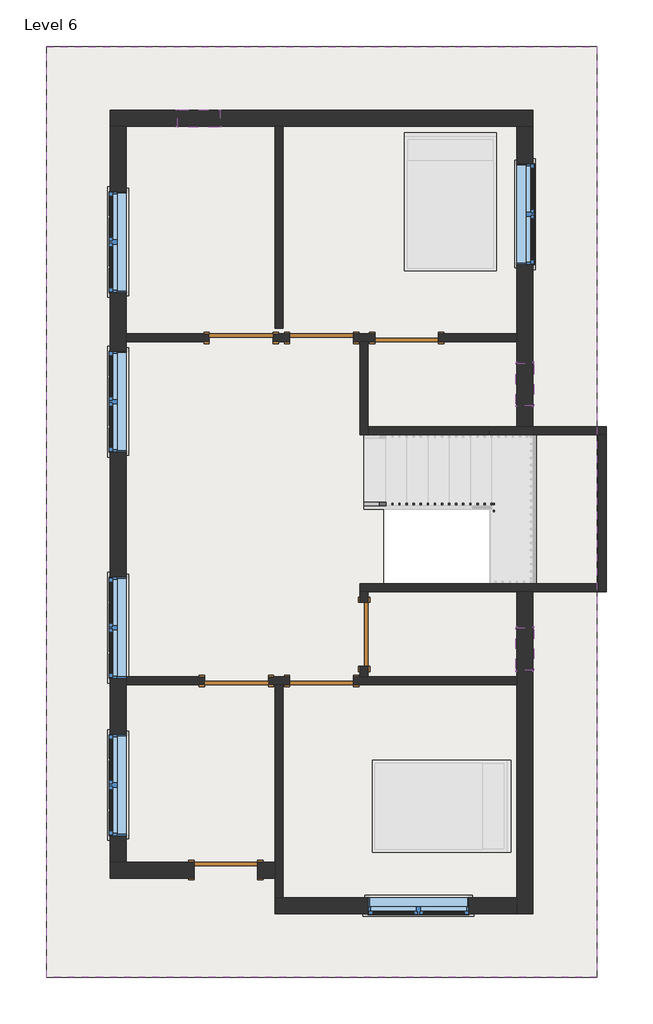
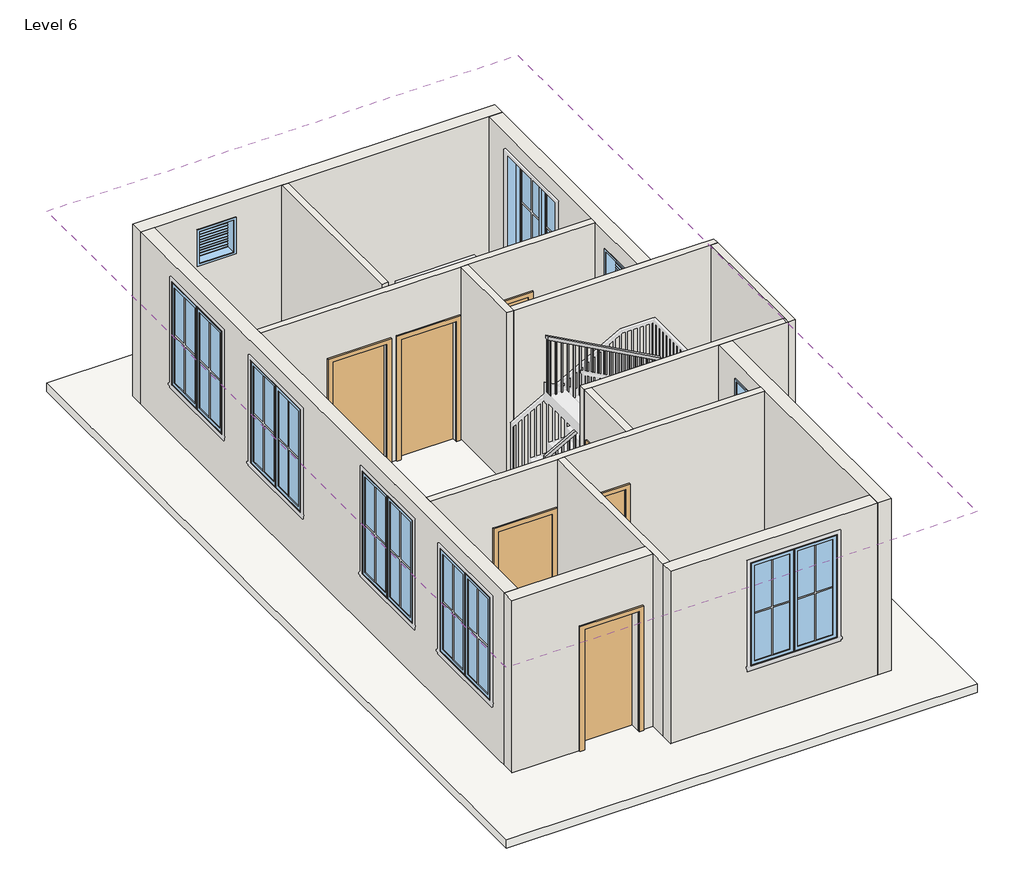
# One storey, part 1 of 2: 15 walls, 9 windows, 7 doors, 2 roofs, 1 railing.
"""IFC4 building model written with IfcOpenShell, lengths in millimetres."""

from ifc_helpers import new_model, si_unit, frame, origin, place, context, project, spatial, polyline, outline, extrude, faceted_brep, transform, mapped, element, save
from components import door_e5f9f3c4, door_305aa2a5, door_0ca8825f, window_9ac97e1a, window_f2d8fef0

model = new_model("IFC4")

# Units and contexts
model_context = context("Model", 3, world=origin())
ifc_project = project(units=[si_unit("LENGTHUNIT", "METRE", prefix="MILLI")], contexts=[model_context])

# Site, building, storey
site = spatial("IfcSite", under=ifc_project)
building = spatial("IfcBuilding", under=site)
storey = spatial("IfcBuildingStorey", under=building, Name="Level 6", Elevation=12801.6)

# Doors
placement = place(None, origin())
door_shape = door_e5f9f3c4(model_context)
element("IfcDoor", 1, ObjectType="Single-Flush : 36\" x 84\"", at=placement, inside=storey, context=model_context, shape_type="MappedRepresentation", body=[
    mapped(door_shape, transform((-2929.7888307, 2238.9017201, 12801.6), x_axis=(1.0, 0.0, 0.0), y_axis=(0.0, 1.0, 0.0), z_axis=(0.0, 0.0, 1.0))),
])
element("IfcDoor", 2, ObjectType="Single-Flush : 36\" x 84\"", at=placement, inside=storey, context=model_context, shape_type="MappedRepresentation", body=[
    mapped(door_shape, transform((-558.0638307, 2238.9017201, 12801.6), x_axis=(-1.0, 0.0, 0.0), y_axis=(0.0, -1.0, 0.0), z_axis=(0.0, 0.0, 1.0))),
])
element("IfcDoor", 3, ObjectType="Single-Flush : 36\" x 84\"", at=placement, inside=storey, context=model_context, shape_type="MappedRepresentation", body=[
    mapped(door_shape, transform((-1167.6638307, -2009.2482799, 12801.6), x_axis=(0.0, -1.0, 0.0), y_axis=(1.0, 0.0, 0.0), z_axis=(0.0, 0.0, 1.0))),
])
element("IfcDoor", 4, ObjectType="Single-Flush : 36\" x 84\"", at=placement, inside=storey, context=model_context, shape_type="MappedRepresentation", body=[
    mapped(door_shape, transform((-1777.2638307, -2675.9982799, 12801.6), x_axis=(-1.0, 0.0, 0.0), y_axis=(0.0, -1.0, 0.0), z_axis=(0.0, 0.0, 1.0))),
])
door_2_shape = door_305aa2a5(model_context)
element("IfcDoor", 5, ObjectType="Single-Flush : 36\" x 84\"", at=placement, inside=storey, context=model_context, shape_type="MappedRepresentation", body=[
    mapped(door_2_shape, transform((-1777.2638307, 2238.9017201, 12801.6), x_axis=(-1.0, 0.0, 0.0), y_axis=(0.0, -1.0, 0.0), z_axis=(0.0, 0.0, 1.0))),
])
element("IfcDoor", 6, ObjectType="Single-Flush : 36\" x 84\"", at=placement, inside=storey, context=model_context, shape_type="MappedRepresentation", body=[
    mapped(door_2_shape, transform((-2996.4638307, -2675.9982799, 12801.6), x_axis=(1.0, 0.0, 0.0), y_axis=(0.0, 1.0, 0.0), z_axis=(0.0, 0.0, 1.0))),
])
door_3_shape = door_0ca8825f(model_context)
element("IfcDoor", 7, ObjectType="Single-Flush : 36\" x 84\"", at=placement, inside=storey, context=model_context, shape_type="MappedRepresentation", body=[
    mapped(door_3_shape, transform((-3148.8638307, -5387.4482799, 12801.6), x_axis=(1.0, 0.0, 0.0), y_axis=(0.0, 1.0, 0.0), z_axis=(0.0, 0.0, 1.0))),
])

# Railing
element("IfcRailing", 8, ObjectType="Handrail - Rectangular", at=placement, inside=storey, context=model_context, shape_type="SolidModel", body=[
    faceted_brep([(-1167.6638307, -116.9482799, 13885.3333333), (-1167.6638307, -116.9482799, 13827.2675836), (-1167.6638307, -167.7482799, 13827.2675836), (-1167.6638307, -167.7482799, 13885.3333333), (591.2861693, -116.9482799, 14859.1464821), (642.0861693, -116.9482799, 14829.2052998), (642.0861693, -167.7482799, 14829.2052998), (591.2861693, -167.7482799, 14859.1464821), (591.2861693, -116.9482799, 14901.3333333), (642.0861693, -116.9482799, 14850.5333333), (642.0861693, -167.7482799, 14850.5333333), (591.2861693, -167.7482799, 14901.3333333), (718.2861693, -116.9482799, 14901.3333333), (718.2861693, -116.9482799, 14850.5333333), (667.4861693, -167.7482799, 14850.5333333), (667.4861693, -167.7482799, 14901.3333333), (718.2861693, -218.5482799, 14901.3333333), (667.4861693, -218.5482799, 14901.3333333), (667.4861693, -269.3482799, 14850.5333333), (718.2861693, -269.3482799, 14850.5333333)], [[[0, 1, 2, 3]], [[1, 0, 4, 5]], [[2, 1, 5, 6]], [[3, 2, 6, 7]], [[0, 3, 7, 4]], [[5, 4, 8, 9]], [[6, 5, 9, 10]], [[7, 6, 10, 11]], [[4, 7, 11, 8]], [[9, 8, 12, 13]], [[10, 9, 13, 14]], [[11, 10, 14, 15]], [[8, 11, 15, 12]], [[16, 17, 18, 19]], [[13, 12, 16, 19]], [[14, 13, 19, 18]], [[15, 14, 18, 17]], [[12, 15, 17, 16]]]),
    faceted_brep([(718.2861693, -218.5482799, 14901.3333333), (718.2861693, -269.3482799, 14850.5333333), (667.4861693, -269.3482799, 14850.5333333), (667.4861693, -218.5482799, 14901.3333333), (718.2861693, -218.5482799, 15042.8310502), (667.4861693, -218.5482799, 15012.7403208), (667.4861693, -269.3482799, 15012.7403208), (718.2861693, -269.3482799, 15042.8310502)], [[[0, 1, 2, 3]], [[4, 5, 6, 7]], [[1, 0, 4, 7]], [[2, 1, 7, 6]], [[3, 2, 6, 5]], [[0, 3, 5, 4]]]),
    faceted_brep([(718.2861693, -269.3482799, 15042.8310502), (667.4861693, -269.3482799, 15012.7403208), (667.4861693, -218.5482799, 15012.7403208), (718.2861693, -218.5482799, 15042.8310502), (-1186.7138307, -269.3482799, 16086.6666667), (-1186.7138307, -218.5482799, 16086.6666667), (-1186.7138307, -218.5482799, 16028.7403208), (-1186.7138307, -269.3482799, 16028.7403208)], [[[0, 1, 2, 3]], [[4, 5, 6, 7]], [[1, 0, 4, 7]], [[2, 1, 7, 6]], [[3, 2, 6, 5]], [[0, 3, 5, 4]]]),
    extrude(outline(polyline([(15995.6855263, -1126.3888307), (16006.1238825, -1145.4388307), (15002.9333333, -1145.4388307), (15002.9333333, -1126.3888307), (15995.6855263, -1126.3888307)])), frame((0.0, -253.4732799, 0.0), z_axis=(0.0, 1.0, 0.0), x_axis=(0.0, 0.0, 1.0)), (0.0, 0.0, 1.0), 19.05),
    extrude(outline(polyline([(15940.0142934, -1024.7888307), (15950.4526496, -1043.8388307), (15002.9333333, -1043.8388307), (15002.9333333, -1024.7888307), (15940.0142934, -1024.7888307)])), frame((0.0, -253.4732799, 0.0), z_axis=(0.0, 1.0, 0.0), x_axis=(0.0, 0.0, 1.0)), (0.0, 0.0, 1.0), 19.05),
    extrude(outline(polyline([(15884.3430606, -923.1888307), (15894.7814167, -942.2388307), (15002.9333333, -942.2388307), (15002.9333333, -923.1888307), (15884.3430606, -923.1888307)])), frame((0.0, -253.4732799, 0.0), z_axis=(0.0, 1.0, 0.0), x_axis=(0.0, 0.0, 1.0)), (0.0, 0.0, 1.0), 19.05),
    extrude(outline(polyline([(15828.6718277, -821.5888307), (15839.1101838, -840.6388307), (14833.6, -840.6388307), (14833.6, -821.5888307), (15828.6718277, -821.5888307)])), frame((0.0, -253.4732799, 0.0), z_axis=(0.0, 1.0, 0.0), x_axis=(0.0, 0.0, 1.0)), (0.0, 0.0, 1.0), 19.05),
    extrude(outline(polyline([(15773.0005948, -719.9888307), (15783.438951, -739.0388307), (14833.6, -739.0388307), (14833.6, -719.9888307), (15773.0005948, -719.9888307)])), frame((0.0, -253.4732799, 0.0), z_axis=(0.0, 1.0, 0.0), x_axis=(0.0, 0.0, 1.0)), (0.0, 0.0, 1.0), 19.05),
    extrude(outline(polyline([(15717.3293619, -618.3888307), (15727.7677181, -637.4388307), (14833.6, -637.4388307), (14833.6, -618.3888307), (15717.3293619, -618.3888307)])), frame((0.0, -253.4732799, 0.0), z_axis=(0.0, 1.0, 0.0), x_axis=(0.0, 0.0, 1.0)), (0.0, 0.0, 1.0), 19.05),
    extrude(outline(polyline([(15661.658129, -516.7888307), (15672.0964852, -535.8388307), (14664.2666667, -535.8388307), (14664.2666667, -516.7888307), (15661.658129, -516.7888307)])), frame((0.0, -253.4732799, 0.0), z_axis=(0.0, 1.0, 0.0), x_axis=(0.0, 0.0, 1.0)), (0.0, 0.0, 1.0), 19.05),
    extrude(outline(polyline([(15605.9868962, -415.1888307), (15616.4252523, -434.2388307), (14664.2666667, -434.2388307), (14664.2666667, -415.1888307), (15605.9868962, -415.1888307)])), frame((0.0, -253.4732799, 0.0), z_axis=(0.0, 1.0, 0.0), x_axis=(0.0, 0.0, 1.0)), (0.0, 0.0, 1.0), 19.05),
    extrude(outline(polyline([(15550.3156633, -313.5888307), (15560.7540195, -332.6388307), (14664.2666667, -332.6388307), (14664.2666667, -313.5888307), (15550.3156633, -313.5888307)])), frame((0.0, -253.4732799, 0.0), z_axis=(0.0, 1.0, 0.0), x_axis=(0.0, 0.0, 1.0)), (0.0, 0.0, 1.0), 19.05),
    extrude(outline(polyline([(15494.6444304, -211.9888307), (15505.0827866, -231.0388307), (14494.9333333, -231.0388307), (14494.9333333, -211.9888307), (15494.6444304, -211.9888307)])), frame((0.0, -253.4732799, 0.0), z_axis=(0.0, 1.0, 0.0), x_axis=(0.0, 0.0, 1.0)), (0.0, 0.0, 1.0), 19.05),
    extrude(outline(polyline([(15438.9731975, -110.3888307), (15449.4115537, -129.4388307), (14494.9333333, -129.4388307), (14494.9333333, -110.3888307), (15438.9731975, -110.3888307)])), frame((0.0, -253.4732799, 0.0), z_axis=(0.0, 1.0, 0.0), x_axis=(0.0, 0.0, 1.0)), (0.0, 0.0, 1.0), 19.05),
    extrude(outline(polyline([(15383.3019647, -8.7888307), (15393.7403208, -27.8388307), (14494.9333333, -27.8388307), (14494.9333333, -8.7888307), (15383.3019647, -8.7888307)])), frame((0.0, -253.4732799, 0.0), z_axis=(0.0, 1.0, 0.0), x_axis=(0.0, 0.0, 1.0)), (0.0, 0.0, 1.0), 19.05),
    extrude(outline(polyline([(15327.6307318, 92.8111693), (15338.0690879, 73.7611693), (14325.6, 73.7611693), (14325.6, 92.8111693), (15327.6307318, 92.8111693)])), frame((0.0, -253.4732799, 0.0), z_axis=(0.0, 1.0, 0.0), x_axis=(0.0, 0.0, 1.0)), (0.0, 0.0, 1.0), 19.05),
    extrude(outline(polyline([(15271.9594989, 194.4111693), (15282.3978551, 175.3611693), (14325.6, 175.3611693), (14325.6, 194.4111693), (15271.9594989, 194.4111693)])), frame((0.0, -253.4732799, 0.0), z_axis=(0.0, 1.0, 0.0), x_axis=(0.0, 0.0, 1.0)), (0.0, 0.0, 1.0), 19.05),
    extrude(outline(polyline([(15216.288266, 296.0111693), (15226.7266222, 276.9611693), (14325.6, 276.9611693), (14325.6, 296.0111693), (15216.288266, 296.0111693)])), frame((0.0, -253.4732799, 0.0), z_axis=(0.0, 1.0, 0.0), x_axis=(0.0, 0.0, 1.0)), (0.0, 0.0, 1.0), 19.05),
    extrude(outline(polyline([(15160.6170332, 397.6111693), (15171.0553893, 378.5611693), (14156.2666667, 378.5611693), (14156.2666667, 397.6111693), (15160.6170332, 397.6111693)])), frame((0.0, -253.4732799, 0.0), z_axis=(0.0, 1.0, 0.0), x_axis=(0.0, 0.0, 1.0)), (0.0, 0.0, 1.0), 19.05),
    extrude(outline(polyline([(15104.9458003, 499.2111693), (15115.3841564, 480.1611693), (14156.2666667, 480.1611693), (14156.2666667, 499.2111693), (15104.9458003, 499.2111693)])), frame((0.0, -253.4732799, 0.0), z_axis=(0.0, 1.0, 0.0), x_axis=(0.0, 0.0, 1.0)), (0.0, 0.0, 1.0), 19.05),
    extrude(outline(polyline([(15049.2745674, 600.8111693), (15059.7129236, 581.7611693), (14156.2666667, 581.7611693), (14156.2666667, 600.8111693), (15049.2745674, 600.8111693)])), frame((0.0, -253.4732799, 0.0), z_axis=(0.0, 1.0, 0.0), x_axis=(0.0, 0.0, 1.0)), (0.0, 0.0, 1.0), 19.05),
    extrude(outline(polyline([(651.6111693, -151.8732799), (651.6111693, -132.8232799), (670.6611693, -132.8232799), (670.6611693, -151.8732799), (651.6111693, -151.8732799)])), frame((0.0, 0.0, 13817.6), z_axis=(0.0, 0.0, 1.0), x_axis=(1.0, 0.0, 0.0)), (0.0, 0.0, 1.0), 1032.9333333),
    extrude(outline(polyline([(14788.7762341, 569.0611693), (14778.2295213, 550.0111693), (13817.6, 550.0111693), (13817.6, 569.0611693), (14788.7762341, 569.0611693)])), frame((0.0, -151.8732799, 0.0), z_axis=(0.0, 1.0, 0.0), x_axis=(0.0, 0.0, 1.0)), (0.0, 0.0, 1.0), 19.05),
    extrude(outline(polyline([(14732.5270991, 467.4611693), (14721.9803863, 448.4111693), (13817.6, 448.4111693), (13817.6, 467.4611693), (14732.5270991, 467.4611693)])), frame((0.0, -151.8732799, 0.0), z_axis=(0.0, 1.0, 0.0), x_axis=(0.0, 0.0, 1.0)), (0.0, 0.0, 1.0), 19.05),
    extrude(outline(polyline([(14676.2779642, 365.8611693), (14665.7312514, 346.8111693), (13648.2666667, 346.8111693), (13648.2666667, 365.8611693), (14676.2779642, 365.8611693)])), frame((0.0, -151.8732799, 0.0), z_axis=(0.0, 1.0, 0.0), x_axis=(0.0, 0.0, 1.0)), (0.0, 0.0, 1.0), 19.05),
    extrude(outline(polyline([(14620.0288292, 264.2611693), (14609.4821164, 245.2111693), (13648.2666667, 245.2111693), (13648.2666667, 264.2611693), (14620.0288292, 264.2611693)])), frame((0.0, -151.8732799, 0.0), z_axis=(0.0, 1.0, 0.0), x_axis=(0.0, 0.0, 1.0)), (0.0, 0.0, 1.0), 19.05),
    extrude(outline(polyline([(14563.7796943, 162.6611693), (14553.2329815, 143.6111693), (13648.2666667, 143.6111693), (13648.2666667, 162.6611693), (14563.7796943, 162.6611693)])), frame((0.0, -151.8732799, 0.0), z_axis=(0.0, 1.0, 0.0), x_axis=(0.0, 0.0, 1.0)), (0.0, 0.0, 1.0), 19.05),
    extrude(outline(polyline([(14507.5305593, 61.0611693), (14496.9838465, 42.0111693), (13478.9333333, 42.0111693), (13478.9333333, 61.0611693), (14507.5305593, 61.0611693)])), frame((0.0, -151.8732799, 0.0), z_axis=(0.0, 1.0, 0.0), x_axis=(0.0, 0.0, 1.0)), (0.0, 0.0, 1.0), 19.05),
    extrude(outline(polyline([(14451.2814244, -40.5388307), (14440.7347116, -59.5888307), (13478.9333333, -59.5888307), (13478.9333333, -40.5388307), (14451.2814244, -40.5388307)])), frame((0.0, -151.8732799, 0.0), z_axis=(0.0, 1.0, 0.0), x_axis=(0.0, 0.0, 1.0)), (0.0, 0.0, 1.0), 19.05),
    extrude(outline(polyline([(14395.0322895, -142.1388307), (14384.4855766, -161.1888307), (13478.9333333, -161.1888307), (13478.9333333, -142.1388307), (14395.0322895, -142.1388307)])), frame((0.0, -151.8732799, 0.0), z_axis=(0.0, 1.0, 0.0), x_axis=(0.0, 0.0, 1.0)), (0.0, 0.0, 1.0), 19.05),
    extrude(outline(polyline([(14338.7831545, -243.7388307), (14328.2364417, -262.7888307), (13309.6, -262.7888307), (13309.6, -243.7388307), (14338.7831545, -243.7388307)])), frame((0.0, -151.8732799, 0.0), z_axis=(0.0, 1.0, 0.0), x_axis=(0.0, 0.0, 1.0)), (0.0, 0.0, 1.0), 19.05),
    extrude(outline(polyline([(14282.5340196, -345.3388307), (14271.9873068, -364.3888307), (13309.6, -364.3888307), (13309.6, -345.3388307), (14282.5340196, -345.3388307)])), frame((0.0, -151.8732799, 0.0), z_axis=(0.0, 1.0, 0.0), x_axis=(0.0, 0.0, 1.0)), (0.0, 0.0, 1.0), 19.05),
    extrude(outline(polyline([(14226.2848846, -446.9388307), (14215.7381718, -465.9888307), (13309.6, -465.9888307), (13309.6, -446.9388307), (14226.2848846, -446.9388307)])), frame((0.0, -151.8732799, 0.0), z_axis=(0.0, 1.0, 0.0), x_axis=(0.0, 0.0, 1.0)), (0.0, 0.0, 1.0), 19.05),
    extrude(outline(polyline([(14170.0357497, -548.5388307), (14159.4890369, -567.5888307), (13140.2666667, -567.5888307), (13140.2666667, -548.5388307), (14170.0357497, -548.5388307)])), frame((0.0, -151.8732799, 0.0), z_axis=(0.0, 1.0, 0.0), x_axis=(0.0, 0.0, 1.0)), (0.0, 0.0, 1.0), 19.05),
    extrude(outline(polyline([(14113.7866147, -650.1388307), (14103.2399019, -669.1888307), (13140.2666667, -669.1888307), (13140.2666667, -650.1388307), (14113.7866147, -650.1388307)])), frame((0.0, -151.8732799, 0.0), z_axis=(0.0, 1.0, 0.0), x_axis=(0.0, 0.0, 1.0)), (0.0, 0.0, 1.0), 19.05),
    extrude(outline(polyline([(14057.5374798, -751.7388307), (14046.990767, -770.7888307), (13140.2666667, -770.7888307), (13140.2666667, -751.7388307), (14057.5374798, -751.7388307)])), frame((0.0, -151.8732799, 0.0), z_axis=(0.0, 1.0, 0.0), x_axis=(0.0, 0.0, 1.0)), (0.0, 0.0, 1.0), 19.05),
    extrude(outline(polyline([(14001.2883448, -853.3388307), (13990.741632, -872.3888307), (12970.9333333, -872.3888307), (12970.9333333, -853.3388307), (14001.2883448, -853.3388307)])), frame((0.0, -151.8732799, 0.0), z_axis=(0.0, 1.0, 0.0), x_axis=(0.0, 0.0, 1.0)), (0.0, 0.0, 1.0), 19.05),
    extrude(outline(polyline([(13945.0392099, -954.9388307), (13934.4924971, -973.9888307), (12970.9333333, -973.9888307), (12970.9333333, -954.9388307), (13945.0392099, -954.9388307)])), frame((0.0, -151.8732799, 0.0), z_axis=(0.0, 1.0, 0.0), x_axis=(0.0, 0.0, 1.0)), (0.0, 0.0, 1.0), 19.05),
    extrude(outline(polyline([(13888.7900749, -1056.5388307), (13878.2433621, -1075.5888307), (12970.9333333, -1075.5888307), (12970.9333333, -1056.5388307), (13888.7900749, -1056.5388307)])), frame((0.0, -151.8732799, 0.0), z_axis=(0.0, 1.0, 0.0), x_axis=(0.0, 0.0, 1.0)), (0.0, 0.0, 1.0), 19.05),
    extrude(outline(polyline([(683.3611693, -234.4232799), (702.4111693, -234.4232799), (702.4111693, -253.4732799), (683.3611693, -253.4732799), (683.3611693, -234.4232799)])), frame((0.0, 0.0, 13986.9333333), z_axis=(0.0, 0.0, 1.0), x_axis=(1.0, 0.0, 0.0)), (0.0, 0.0, 1.0), 863.6),
    extrude(outline(polyline([(683.3611693, -151.8732799), (683.3611693, -132.8232799), (702.4111693, -132.8232799), (702.4111693, -151.8732799), (683.3611693, -151.8732799)])), frame((0.0, 0.0, 13986.9333333), z_axis=(0.0, 0.0, 1.0), x_axis=(1.0, 0.0, 0.0)), (0.0, 0.0, 1.0), 863.6),
    extrude(outline(polyline([(16018.3019647, -1167.6638307), (16028.7403208, -1186.7138307), (15002.9333333, -1186.7138307), (15002.9333333, -1167.6638307), (16018.3019647, -1167.6638307)])), frame((0.0, -253.4732799, 0.0), z_axis=(0.0, 1.0, 0.0), x_axis=(0.0, 0.0, 1.0)), (0.0, 0.0, 1.0), 19.05),
    extrude(outline(polyline([(13837.8142964, -1148.6138307), (13827.2675836, -1167.6638307), (12970.9333333, -1167.6638307), (12970.9333333, -1148.6138307), (13837.8142964, -1148.6138307)])), frame((0.0, -151.8732799, 0.0), z_axis=(0.0, 1.0, 0.0), x_axis=(0.0, 0.0, 1.0)), (0.0, 0.0, 1.0), 19.05),
])

# Roofs
element("IfcRoof", 9, ObjectType="ROOF 6\"", at=placement, inside=storey, context=model_context, shape_type="SweptSolid", body=[
    extrude(outline(polyline([(-5720.6138307, -6924.1482799), (-5720.6138307, 6410.8517201), (2166.0861693, 6410.8517201), (2166.0861693, -6924.1482799), (-5720.6138307, -6924.1482799)]), holes=[polyline([(1251.6861693, -1285.3482799), (1251.6861693, 899.0517201), (-881.9138307, 899.0517201), (-881.9138307, -1285.3482799), (1251.6861693, -1285.3482799)])]), frame((0.0, 0.0, 12649.2), z_axis=(0.0, 0.0, 1.0), x_axis=(1.0, 0.0, 0.0)), (0.0, 0.0, 1.0), 152.4),
])
element("IfcRoof", 10, ObjectType="ROOF 6\"", at=placement, inside=storey, context=model_context, shape_type="SweptSolid", body=[
    extrude(outline(polyline([(-5720.6138307, -6924.1482799), (-5720.6138307, 6410.8517201), (2166.0861693, 6410.8517201), (2166.0861693, -6924.1482799), (-5720.6138307, -6924.1482799)]), holes=[polyline([(1251.6861693, -1285.3482799), (1251.6861693, 899.0517201), (-881.9138307, 899.0517201), (-881.9138307, -1285.3482799), (1251.6861693, -1285.3482799)])]), frame((0.0, 0.0, 15849.6), z_axis=(0.0, 0.0, 1.0), x_axis=(1.0, 0.0, 0.0)), (0.0, 0.0, 1.0), 152.4),
])

# Walls
element("IfcWall", 11, ObjectType="WALL 4.5\"", at=placement, inside=storey, context=model_context, shape_type="SweptSolid", body=[
    extrude(outline(polyline([(-2444.0138307, 2372.2517201), (-2444.0138307, 5267.8517201), (-2329.7138307, 5267.8517201), (-2329.7138307, 2372.2517201), (-2444.0138307, 2372.2517201)])), frame((0.0, 0.0, 12801.6), z_axis=(0.0, 0.0, 1.0), x_axis=(1.0, 0.0, 0.0)), (0.0, 0.0, 1.0), 3048.0),
])
element("IfcWall", 12, ObjectType="WALL 4.5\"", at=placement, inside=storey, context=model_context, shape_type="Brep", body=[
    faceted_brep([(-1320.0638307, 2181.7517201, 12801.6), (-1224.8138307, 2181.7517201, 12801.6), (-1110.5138307, 2181.7517201, 12801.6), (-1015.2638307, 2181.7517201, 12801.6), (-1015.2638307, 2181.7517201, 14935.2), (-100.8638307, 2181.7517201, 14935.2), (-100.8638307, 2181.7517201, 12801.6), (1023.0861693, 2181.7517201, 12801.6), (1023.0861693, 2181.7517201, 15849.6), (-1110.5138307, 2181.7517201, 15849.6), (-1224.8138307, 2181.7517201, 15849.6), (-4577.6138307, 2181.7517201, 15849.6), (-4577.6138307, 2181.7517201, 12801.6), (-3386.9888307, 2181.7517201, 12801.6), (-3386.9888307, 2181.7517201, 14935.2), (-2472.5888307, 2181.7517201, 14935.2), (-2472.5888307, 2181.7517201, 12801.6), (-2234.4638307, 2181.7517201, 12801.6), (-2234.4638307, 2181.7517201, 14935.2), (-1320.0638307, 2181.7517201, 14935.2), (-1015.2638307, 2296.0517201, 14935.2), (-1015.2638307, 2296.0517201, 12801.6), (-1320.0638307, 2296.0517201, 12801.6), (-1320.0638307, 2296.0517201, 14935.2), (-2234.4638307, 2296.0517201, 14935.2), (-2234.4638307, 2296.0517201, 12801.6), (-2472.5888307, 2296.0517201, 12801.6), (-2472.5888307, 2296.0517201, 14935.2), (-3386.9888307, 2296.0517201, 14935.2), (-3386.9888307, 2296.0517201, 12801.6), (-4577.6138307, 2296.0517201, 12801.6), (-4577.6138307, 2296.0517201, 15849.6), (1023.0861693, 2296.0517201, 15849.6), (1023.0861693, 2296.0517201, 12801.6), (-100.8638307, 2296.0517201, 12801.6), (-100.8638307, 2296.0517201, 14935.2)], [[[0, 1, 2, 3, 4, 5, 6, 7, 8, 9, 10, 11, 12, 13, 14, 15, 16, 17, 18, 19]], [[20, 21, 22, 23, 24, 25, 26, 27, 28, 29, 30, 31, 32, 33, 34, 35]], [[13, 12, 30, 29]], [[26, 25, 17, 16]], [[34, 33, 7, 6]], [[22, 21, 3, 2, 1, 0]], [[8, 7, 33, 32]], [[12, 11, 31, 30]], [[27, 26, 16, 15]], [[28, 27, 15, 14]], [[29, 28, 14, 13]], [[18, 17, 25, 24]], [[19, 18, 24, 23]], [[0, 19, 23, 22]], [[4, 3, 21, 20]], [[5, 4, 20, 35]], [[6, 5, 35, 34]], [[11, 10, 9, 8, 32, 31]]]),
])
element("IfcWall", 13, ObjectType="WALL 4.5\"", at=placement, inside=storey, context=model_context, shape_type="Brep", body=[
    faceted_brep([(-1224.8138307, 2181.7517201, 12801.6), (-1224.8138307, 848.2517201, 12801.6), (-1224.8138307, 848.2517201, 15849.6), (-1224.8138307, 2181.7517201, 15849.6), (-1110.5138307, 2181.7517201, 12801.6), (-1110.5138307, 2181.7517201, 15849.6), (-1110.5138307, 962.5517201, 15849.6), (-1110.5138307, 848.2517201, 15849.6), (-1110.5138307, 848.2517201, 12801.6), (-1110.5138307, 962.5517201, 12801.6)], [[[0, 1, 2, 3]], [[4, 5, 6, 7, 8, 9]], [[1, 0, 4, 9, 8]], [[0, 3, 5, 4]], [[2, 1, 8, 7]], [[3, 2, 7, 6, 5]]]),
])
element("IfcWall", 14, ObjectType="WALL 4.5\"", at=placement, inside=storey, context=model_context, shape_type="Brep", body=[
    faceted_brep([(-1110.5138307, 848.2517201, 12801.6), (2191.4861693, 848.2517201, 12801.6), (2305.7861693, 848.2517201, 12801.6), (2305.7861693, 848.2517201, 15849.6), (2191.4861693, 848.2517201, 15849.6), (-1110.5138307, 848.2517201, 15849.6), (-1110.5138307, 962.5517201, 12801.6), (-1110.5138307, 962.5517201, 15849.6), (1023.0861693, 962.5517201, 15849.6), (1251.6861693, 962.5517201, 15849.6), (2305.7861693, 962.5517201, 15849.6), (2305.7861693, 962.5517201, 12801.6), (1251.6861693, 962.5517201, 12801.6), (1023.0861693, 962.5517201, 12801.6)], [[[0, 1, 2, 3, 4, 5]], [[6, 7, 8, 9, 10, 11, 12, 13]], [[2, 1, 0, 6, 13, 12, 11]], [[5, 4, 3, 10, 9, 8, 7]], [[0, 5, 7, 6]], [[3, 2, 11, 10]]]),
])
element("IfcWall", 15, ObjectType="WALL 4.5\"", at=placement, inside=storey, context=model_context, shape_type="Brep", body=[
    faceted_brep([(2191.4861693, 848.2517201, 12801.6), (2191.4861693, -1285.3482799, 12801.6), (2191.4861693, -1399.6482799, 12801.6), (2191.4861693, -1399.6482799, 15849.6), (2191.4861693, -1285.3482799, 15849.6), (2191.4861693, 848.2517201, 15849.6), (2305.7861693, 848.2517201, 12801.6), (2305.7861693, 848.2517201, 15849.6), (2305.7861693, -1399.6482799, 15849.6), (2305.7861693, -1399.6482799, 12801.6)], [[[0, 1, 2, 3, 4, 5]], [[6, 7, 8, 9]], [[2, 1, 0, 6, 9]], [[5, 4, 3, 8, 7]], [[0, 5, 7, 6]], [[3, 2, 9, 8]]]),
])
element("IfcWall", 16, ObjectType="WALL 4.5\"", at=placement, inside=storey, context=model_context, shape_type="Brep", body=[
    faceted_brep([(2191.4861693, -1285.3482799, 12801.6), (-1224.8138307, -1285.3482799, 12801.6), (-1224.8138307, -1285.3482799, 15849.6), (-881.9138307, -1285.3482799, 15849.6), (1251.6861693, -1285.3482799, 15849.6), (2166.0861693, -1285.3482799, 15849.6), (2191.4861693, -1285.3482799, 15849.6), (2191.4861693, -1399.6482799, 12801.6), (2191.4861693, -1399.6482799, 15849.6), (2166.0861693, -1399.6482799, 15849.6), (1251.6861693, -1399.6482799, 15849.6), (1023.0861693, -1399.6482799, 15849.6), (-1110.5138307, -1399.6482799, 15849.6), (-1224.8138307, -1399.6482799, 15849.6), (-1224.8138307, -1399.6482799, 12801.6), (-1110.5138307, -1399.6482799, 12801.6), (1023.0861693, -1399.6482799, 12801.6), (1251.6861693, -1399.6482799, 12801.6)], [[[0, 1, 2, 3, 4, 5, 6]], [[7, 8, 9, 10, 11, 12, 13, 14, 15, 16, 17]], [[1, 0, 7, 17, 16, 15, 14]], [[0, 6, 8, 7]], [[2, 1, 14, 13]], [[6, 5, 9, 8]], [[5, 4, 3, 2, 13, 12, 11, 10, 9]]]),
])
element("IfcWall", 17, ObjectType="WALL 4.5\"", at=placement, inside=storey, context=model_context, shape_type="SweptSolid", body=[
    extrude(outline(polyline([(-2466.4482799, 14935.2), (-2466.4482799, 12801.6), (-2618.8482799, 12801.6), (-2618.8482799, 15849.6), (-1399.6482799, 15849.6), (-1399.6482799, 12801.6), (-1552.0482799, 12801.6), (-1552.0482799, 14935.2), (-2466.4482799, 14935.2)])), frame((-1224.8138307, 0.0, 0.0), z_axis=(1.0, 0.0, 0.0), x_axis=(0.0, 1.0, 0.0)), (0.0, 0.0, 1.0), 114.3),
])
element("IfcWall", 18, ObjectType="WALL 4.5\"", at=placement, inside=storey, context=model_context, shape_type="Brep", body=[
    faceted_brep([(-2234.4638307, -2618.8482799, 12801.6), (-2539.2638307, -2618.8482799, 12801.6), (-2539.2638307, -2618.8482799, 14935.2), (-3453.6638307, -2618.8482799, 14935.2), (-3453.6638307, -2618.8482799, 12801.6), (-4577.6138307, -2618.8482799, 12801.6), (-4577.6138307, -2618.8482799, 15849.6), (-1224.8138307, -2618.8482799, 15849.6), (-1110.5138307, -2618.8482799, 15849.6), (1023.0861693, -2618.8482799, 15849.6), (1023.0861693, -2618.8482799, 12801.6), (-1110.5138307, -2618.8482799, 12801.6), (-1224.8138307, -2618.8482799, 12801.6), (-1320.0638307, -2618.8482799, 12801.6), (-1320.0638307, -2618.8482799, 14935.2), (-2234.4638307, -2618.8482799, 14935.2), (-2539.2638307, -2733.1482799, 14935.2), (-2539.2638307, -2733.1482799, 12801.6), (-2444.0138307, -2733.1482799, 12801.6), (-2329.7138307, -2733.1482799, 12801.6), (-2234.4638307, -2733.1482799, 12801.6), (-2234.4638307, -2733.1482799, 14935.2), (-1320.0638307, -2733.1482799, 14935.2), (-1320.0638307, -2733.1482799, 12801.6), (1023.0861693, -2733.1482799, 12801.6), (1023.0861693, -2733.1482799, 15849.6), (-2329.7138307, -2733.1482799, 15849.6), (-2444.0138307, -2733.1482799, 15849.6), (-4577.6138307, -2733.1482799, 15849.6), (-4577.6138307, -2733.1482799, 12801.6), (-3453.6638307, -2733.1482799, 12801.6), (-3453.6638307, -2733.1482799, 14935.2)], [[[0, 1, 2, 3, 4, 5, 6, 7, 8, 9, 10, 11, 12, 13, 14, 15]], [[16, 17, 18, 19, 20, 21, 22, 23, 24, 25, 26, 27, 28, 29, 30, 31]], [[13, 12, 11, 10, 24, 23]], [[30, 29, 5, 4]], [[20, 19, 18, 17, 1, 0]], [[10, 9, 25, 24]], [[6, 5, 29, 28]], [[21, 20, 0, 15]], [[22, 21, 15, 14]], [[23, 22, 14, 13]], [[2, 1, 17, 16]], [[3, 2, 16, 31]], [[4, 3, 31, 30]], [[9, 8, 7, 6, 28, 27, 26, 25]]]),
])
element("IfcWall", 19, ObjectType="WALL 4.5\"", at=placement, inside=storey, context=model_context, shape_type="Brep", body=[
    faceted_brep([(-2329.7138307, -5781.1482799, 12801.6), (-2329.7138307, -2733.1482799, 12801.6), (-2329.7138307, -2733.1482799, 15849.6), (-2329.7138307, -5781.1482799, 15849.6), (-2444.0138307, -5781.1482799, 12801.6), (-2444.0138307, -5781.1482799, 15849.6), (-2444.0138307, -5501.7482799, 15849.6), (-2444.0138307, -5273.1482799, 15849.6), (-2444.0138307, -2733.1482799, 15849.6), (-2444.0138307, -2733.1482799, 12801.6), (-2444.0138307, -5273.1482799, 12801.6), (-2444.0138307, -5501.7482799, 12801.6)], [[[0, 1, 2, 3]], [[4, 5, 6, 7, 8, 9, 10, 11]], [[1, 0, 4, 11, 10, 9]], [[0, 3, 5, 4]], [[2, 1, 9, 8]], [[3, 2, 8, 7, 6, 5]]]),
])
element("IfcWall", 20, ObjectType="WALL 9\"", at=placement, inside=storey, context=model_context, shape_type="Brep", body=[
    faceted_brep([(-4806.2138307, 5267.8517201, 12801.6), (-4577.6138307, 5267.8517201, 12801.6), (-2444.0138307, 5267.8517201, 12801.6), (-2329.7138307, 5267.8517201, 12801.6), (1023.0861693, 5267.8517201, 12801.6), (1251.6861693, 5267.8517201, 12801.6), (1251.6861693, 5267.8517201, 15849.6), (1023.0861693, 5267.8517201, 15849.6), (-2329.7138307, 5267.8517201, 15849.6), (-2444.0138307, 5267.8517201, 15849.6), (-4577.6138307, 5267.8517201, 15849.6), (-4806.2138307, 5267.8517201, 15849.6), (-3844.1888307, 5267.8517201, 15544.8), (-3234.5888307, 5267.8517201, 15544.8), (-3234.5888307, 5267.8517201, 14935.2), (-3844.1888307, 5267.8517201, 14935.2), (-4806.2138307, 5496.4517201, 12801.6), (-4806.2138307, 5496.4517201, 15849.6), (1251.6861693, 5496.4517201, 15849.6), (1251.6861693, 5496.4517201, 12801.6), (-3844.1888307, 5496.4517201, 15544.8), (-3844.1888307, 5496.4517201, 14935.2), (-3234.5888307, 5496.4517201, 14935.2), (-3234.5888307, 5496.4517201, 15544.8)], [[[0, 1, 2, 3, 4, 5, 6, 7, 8, 9, 10, 11], [12, 13, 14, 15]], [[16, 17, 18, 19], [20, 21, 22, 23]], [[5, 4, 3, 2, 1, 0, 16, 19]], [[6, 5, 19, 18]], [[0, 11, 17, 16]], [[21, 20, 12, 15]], [[22, 21, 15, 14]], [[23, 22, 14, 13]], [[20, 23, 13, 12]], [[11, 10, 9, 8, 7, 6, 18, 17]]]),
])
element("IfcWall", 21, ObjectType="WALL 9\"", at=placement, inside=storey, context=model_context, shape_type="Brep", body=[
    faceted_brep([(1023.0861693, 5267.8517201, 12801.6), (1023.0861693, 2296.0517201, 12801.6), (1023.0861693, 2181.7517201, 12801.6), (1023.0861693, 962.5517201, 12801.6), (1023.0861693, 962.5517201, 15849.6), (1023.0861693, 2181.7517201, 15849.6), (1023.0861693, 2296.0517201, 15849.6), (1023.0861693, 5267.8517201, 15849.6), (1023.0861693, 3286.6517201, 15544.8), (1023.0861693, 3286.6517201, 13716.0), (1023.0861693, 4734.4517201, 13716.0), (1023.0861693, 4734.4517201, 15544.8), (1023.0861693, 1876.9517201, 15544.8), (1023.0861693, 1267.3517201, 15544.8), (1023.0861693, 1267.3517201, 14935.2), (1023.0861693, 1876.9517201, 14935.2), (1251.6861693, 5267.8517201, 12801.6), (1251.6861693, 5267.8517201, 15849.6), (1251.6861693, 962.5517201, 15849.6), (1251.6861693, 962.5517201, 12801.6), (1251.6861693, 3286.6517201, 15544.8), (1251.6861693, 4734.4517201, 15544.8), (1251.6861693, 4734.4517201, 13716.0), (1251.6861693, 3286.6517201, 13716.0), (1251.6861693, 1876.9517201, 15544.8), (1251.6861693, 1876.9517201, 14935.2), (1251.6861693, 1267.3517201, 14935.2), (1251.6861693, 1267.3517201, 15544.8)], [[[0, 1, 2, 3, 4, 5, 6, 7], [8, 9, 10, 11], [12, 13, 14, 15]], [[16, 17, 18, 19], [20, 21, 22, 23], [24, 25, 26, 27]], [[3, 2, 1, 0, 16, 19]], [[0, 7, 17, 16]], [[4, 3, 19, 18]], [[9, 8, 20, 23]], [[10, 9, 23, 22]], [[11, 10, 22, 21]], [[8, 11, 21, 20]], [[25, 24, 12, 15]], [[26, 25, 15, 14]], [[27, 26, 14, 13]], [[24, 27, 13, 12]], [[7, 6, 5, 4, 18, 17]]]),
])
element("IfcWall", 22, ObjectType="WALL 9\"", at=placement, inside=storey, context=model_context, shape_type="Brep", body=[
    faceted_brep([(1023.0861693, -1399.6482799, 12801.6), (1023.0861693, -2618.8482799, 12801.6), (1023.0861693, -2733.1482799, 12801.6), (1023.0861693, -5781.1482799, 12801.6), (1023.0861693, -6009.7482799, 12801.6), (1023.0861693, -6009.7482799, 15849.6), (1023.0861693, -5781.1482799, 15849.6), (1023.0861693, -2733.1482799, 15849.6), (1023.0861693, -2618.8482799, 15849.6), (1023.0861693, -1399.6482799, 15849.6), (1023.0861693, -1913.9982799, 15544.8), (1023.0861693, -2523.5982799, 15544.8), (1023.0861693, -2523.5982799, 14935.2), (1023.0861693, -1913.9982799, 14935.2), (1251.6861693, -1399.6482799, 12801.6), (1251.6861693, -1399.6482799, 15849.6), (1251.6861693, -6009.7482799, 15849.6), (1251.6861693, -6009.7482799, 12801.6), (1251.6861693, -1913.9982799, 15544.8), (1251.6861693, -1913.9982799, 14935.2), (1251.6861693, -2523.5982799, 14935.2), (1251.6861693, -2523.5982799, 15544.8)], [[[0, 1, 2, 3, 4, 5, 6, 7, 8, 9], [10, 11, 12, 13]], [[14, 15, 16, 17], [18, 19, 20, 21]], [[4, 3, 2, 1, 0, 14, 17]], [[5, 4, 17, 16]], [[0, 9, 15, 14]], [[19, 18, 10, 13]], [[20, 19, 13, 12]], [[21, 20, 12, 11]], [[18, 21, 11, 10]], [[9, 8, 7, 6, 5, 16, 15]]]),
])
element("IfcWall", 23, ObjectType="WALL 9\"", at=placement, inside=storey, context=model_context, shape_type="Brep", body=[
    faceted_brep([(1023.0861693, -5781.1482799, 12801.6), (-2329.7138307, -5781.1482799, 12801.6), (-2444.0138307, -5781.1482799, 12801.6), (-2444.0138307, -5781.1482799, 15849.6), (-2329.7138307, -5781.1482799, 15849.6), (1023.0861693, -5781.1482799, 15849.6), (-1110.5138307, -5781.1482799, 15544.8), (-1110.5138307, -5781.1482799, 13716.0), (337.2861693, -5781.1482799, 13716.0), (337.2861693, -5781.1482799, 15544.8), (1023.0861693, -6009.7482799, 12801.6), (1023.0861693, -6009.7482799, 15849.6), (-2444.0138307, -6009.7482799, 15849.6), (-2444.0138307, -6009.7482799, 12801.6), (-1110.5138307, -6009.7482799, 15544.8), (337.2861693, -6009.7482799, 15544.8), (337.2861693, -6009.7482799, 13716.0), (-1110.5138307, -6009.7482799, 13716.0)], [[[0, 1, 2, 3, 4, 5], [6, 7, 8, 9]], [[10, 11, 12, 13], [14, 15, 16, 17]], [[2, 1, 0, 10, 13]], [[0, 5, 11, 10]], [[3, 2, 13, 12]], [[7, 6, 14, 17]], [[8, 7, 17, 16]], [[9, 8, 16, 15]], [[6, 9, 15, 14]], [[5, 4, 3, 12, 11]]]),
])
element("IfcWall", 24, ObjectType="WALL 9\"", at=placement, inside=storey, context=model_context, shape_type="Brep", body=[
    faceted_brep([(-2691.6638307, -5501.7482799, 14935.2), (-2691.6638307, -5501.7482799, 12801.6), (-2444.0138307, -5501.7482799, 12801.6), (-2444.0138307, -5501.7482799, 15849.6), (-4806.2138307, -5501.7482799, 15849.6), (-4806.2138307, -5501.7482799, 12801.6), (-3606.0638307, -5501.7482799, 12801.6), (-3606.0638307, -5501.7482799, 14935.2), (-2444.0138307, -5273.1482799, 12801.6), (-2691.6638307, -5273.1482799, 12801.6), (-2691.6638307, -5273.1482799, 14935.2), (-3606.0638307, -5273.1482799, 14935.2), (-3606.0638307, -5273.1482799, 12801.6), (-4577.6138307, -5273.1482799, 12801.6), (-4806.2138307, -5273.1482799, 12801.6), (-4806.2138307, -5273.1482799, 15849.6), (-4577.6138307, -5273.1482799, 15849.6), (-2444.0138307, -5273.1482799, 15849.6)], [[[0, 1, 2, 3, 4, 5, 6, 7]], [[8, 9, 10, 11, 12, 13, 14, 15, 16, 17]], [[6, 5, 14, 13, 12]], [[2, 1, 9, 8]], [[5, 4, 15, 14]], [[3, 2, 8, 17]], [[10, 9, 1, 0]], [[11, 10, 0, 7]], [[12, 11, 7, 6]], [[4, 3, 17, 16, 15]]]),
])
element("IfcWall", 25, ObjectType="WALL 9\"", at=placement, inside=storey, context=model_context, shape_type="Brep", body=[
    faceted_brep([(-4577.6138307, -5273.1482799, 12801.6), (-4577.6138307, -2733.1482799, 12801.6), (-4577.6138307, -2618.8482799, 12801.6), (-4577.6138307, 2181.7517201, 12801.6), (-4577.6138307, 2296.0517201, 12801.6), (-4577.6138307, 5267.8517201, 12801.6), (-4577.6138307, 5267.8517201, 15849.6), (-4577.6138307, 2296.0517201, 15849.6), (-4577.6138307, 2181.7517201, 15849.6), (-4577.6138307, -2618.8482799, 15849.6), (-4577.6138307, -2733.1482799, 15849.6), (-4577.6138307, -5273.1482799, 15849.6), (-4577.6138307, -3444.3482799, 15544.8), (-4577.6138307, -3444.3482799, 13716.0), (-4577.6138307, -4892.1482799, 13716.0), (-4577.6138307, -4892.1482799, 15544.8), (-4577.6138307, -1190.0982799, 15544.8), (-4577.6138307, -1190.0982799, 13716.0), (-4577.6138307, -2637.8982799, 13716.0), (-4577.6138307, -2637.8982799, 15544.8), (-4577.6138307, 4334.4017201, 15544.8), (-4577.6138307, 4334.4017201, 13716.0), (-4577.6138307, 2886.6017201, 13716.0), (-4577.6138307, 2886.6017201, 15544.8), (-4577.6138307, 2048.4017201, 15544.8), (-4577.6138307, 2048.4017201, 13716.0), (-4577.6138307, 600.6017201, 13716.0), (-4577.6138307, 600.6017201, 15544.8), (-4806.2138307, -5273.1482799, 12801.6), (-4806.2138307, -5273.1482799, 15849.6), (-4806.2138307, 5267.8517201, 15849.6), (-4806.2138307, 5267.8517201, 12801.6), (-4806.2138307, -3444.3482799, 15544.8), (-4806.2138307, -4892.1482799, 15544.8), (-4806.2138307, -4892.1482799, 13716.0), (-4806.2138307, -3444.3482799, 13716.0), (-4806.2138307, -1190.0982799, 15544.8), (-4806.2138307, -2637.8982799, 15544.8), (-4806.2138307, -2637.8982799, 13716.0), (-4806.2138307, -1190.0982799, 13716.0), (-4806.2138307, 4334.4017201, 15544.8), (-4806.2138307, 2886.6017201, 15544.8), (-4806.2138307, 2886.6017201, 13716.0), (-4806.2138307, 4334.4017201, 13716.0), (-4806.2138307, 2048.4017201, 15544.8), (-4806.2138307, 600.6017201, 15544.8), (-4806.2138307, 600.6017201, 13716.0), (-4806.2138307, 2048.4017201, 13716.0)], [[[0, 1, 2, 3, 4, 5, 6, 7, 8, 9, 10, 11], [12, 13, 14, 15], [16, 17, 18, 19], [20, 21, 22, 23], [24, 25, 26, 27]], [[28, 29, 30, 31], [32, 33, 34, 35], [36, 37, 38, 39], [40, 41, 42, 43], [44, 45, 46, 47]], [[5, 4, 3, 2, 1, 0, 28, 31]], [[6, 5, 31, 30]], [[0, 11, 29, 28]], [[13, 12, 32, 35]], [[14, 13, 35, 34]], [[15, 14, 34, 33]], [[12, 15, 33, 32]], [[17, 16, 36, 39]], [[18, 17, 39, 38]], [[19, 18, 38, 37]], [[16, 19, 37, 36]], [[21, 20, 40, 43]], [[22, 21, 43, 42]], [[23, 22, 42, 41]], [[20, 23, 41, 40]], [[25, 24, 44, 47]], [[26, 25, 47, 46]], [[27, 26, 46, 45]], [[24, 27, 45, 44]], [[11, 10, 9, 8, 7, 6, 30, 29]]]),
])

# Windows
window_shape = window_9ac97e1a(model_context)
element("IfcWindow", 26, ObjectType="Window-Casement-Double : 57\" x 72\"", at=placement, inside=storey, context=model_context, shape_type="MappedRepresentation", body=[
    mapped(window_shape, transform((-4691.9138307, -4168.2482799, 12801.6), x_axis=(0.0, 1.0, 0.0), y_axis=(-1.0, 0.0, 0.0), z_axis=(0.0, 0.0, 1.0))),
])
element("IfcWindow", 27, ObjectType="Window-Casement-Double : 57\" x 72\"", at=placement, inside=storey, context=model_context, shape_type="MappedRepresentation", body=[
    mapped(window_shape, transform((-4691.9138307, -1913.9982799, 12801.6), x_axis=(0.0, 1.0, 0.0), y_axis=(-1.0, 0.0, 0.0), z_axis=(0.0, 0.0, 1.0))),
])
element("IfcWindow", 28, ObjectType="Window-Casement-Double : 57\" x 72\"", at=placement, inside=storey, context=model_context, shape_type="MappedRepresentation", body=[
    mapped(window_shape, transform((-386.6138307, -5895.4482799, 12801.6), x_axis=(-1.0, 0.0, 0.0), y_axis=(0.0, -1.0, 0.0), z_axis=(0.0, 0.0, 1.0))),
])
element("IfcWindow", 29, ObjectType="Window-Casement-Double : 57\" x 72\"", at=placement, inside=storey, context=model_context, shape_type="MappedRepresentation", body=[
    mapped(window_shape, transform((1137.3861693, 4010.5517201, 12801.6), x_axis=(0.0, -1.0, 0.0), y_axis=(1.0, 0.0, 0.0), z_axis=(0.0, 0.0, 1.0))),
])
element("IfcWindow", 30, ObjectType="Window-Casement-Double : 57\" x 72\"", at=placement, inside=storey, context=model_context, shape_type="MappedRepresentation", body=[
    mapped(window_shape, transform((-4691.9138307, 3610.5017201, 12801.6), x_axis=(0.0, 1.0, 0.0), y_axis=(-1.0, 0.0, 0.0), z_axis=(0.0, 0.0, 1.0))),
])
element("IfcWindow", 31, ObjectType="Window-Casement-Double : 57\" x 72\"", at=placement, inside=storey, context=model_context, shape_type="MappedRepresentation", body=[
    mapped(window_shape, transform((-4691.9138307, 1324.5017201, 12801.6), x_axis=(0.0, 1.0, 0.0), y_axis=(-1.0, 0.0, 0.0), z_axis=(0.0, 0.0, 1.0))),
])
window_2_shape = window_f2d8fef0(model_context)
element("IfcWindow", 32, ObjectType="Window-Louvers : 24\" x 24\"", at=placement, inside=storey, context=model_context, shape_type="MappedRepresentation", body=[
    mapped(window_2_shape, transform((1143.7361693, 1572.1517201, 14020.8), x_axis=(0.0, -1.0, 0.0), y_axis=(1.0, 0.0, 0.0), z_axis=(0.0, 0.0, 1.0))),
])
element("IfcWindow", 33, ObjectType="Window-Louvers : 24\" x 24\"", at=placement, inside=storey, context=model_context, shape_type="MappedRepresentation", body=[
    mapped(window_2_shape, transform((-3539.3888307, 5388.5017201, 14020.8), x_axis=(1.0, 0.0, 0.0), y_axis=(0.0, 1.0, 0.0), z_axis=(0.0, 0.0, 1.0))),
])
element("IfcWindow", 34, ObjectType="Window-Louvers : 24\" x 24\"", at=placement, inside=storey, context=model_context, shape_type="MappedRepresentation", body=[
    mapped(window_2_shape, transform((1143.7361693, -2218.7982799, 14020.8), x_axis=(0.0, -1.0, 0.0), y_axis=(1.0, 0.0, 0.0), z_axis=(0.0, 0.0, 1.0))),
])

save(model, "model.ifc")

# Revit data of these elements
# Type "Single-Flush : 36\" x 84\""
#   Type Mark = "1"
#   Construction Type Id = "MDOOR"
#   Assembly Code = "C1020"
#   Analytic Construction = "Metal"
#   Thickness = 0' - 2"
#   Heat Transfer Coefficient (U) = 0.651978 BTU/(h·ft²·°F)
#   Height = 7' - 0"
#   Trim Projection Ext = 0' - 1"
#   Trim Projection Int = 0' - 1"
#   Trim Width = 0' - 3"
#   Width = 3' - 0"
#   Define Thermal Properties by = 1
#   Define Thermal Properties by = 1
#   Door Material = Door - Panel
#   Frame Material = Door - Frame
#   Visual Light Transmittance = 0
#   Solar Heat Gain Coefficient = 0
#   Function = (empty or 0)
#   Wall Closure = (empty or 0)
# Type "Handrail - Rectangular"
#   Assembly Code = "C2010400"
#   built-in parameter 1008612 = 0.0416667 (stored number, unit not read)
#   built-in parameter 1008611 = 0.0416667 (stored number, unit not read)
#   built-in parameter 1008609 = 0.333333 (stored number, unit not read)
#   built-in parameter 1008604 = 0.166667 (stored number, unit not read)
#   built-in parameter 1008603 = 0.166667 (stored number, unit not read)
#   Railing Height = 3' - 0"
#   built-in parameter 1008630 = 2
#   built-in parameter 1008610 = 2
#   built-in parameter 1008618 = Baluster - Square : 3/4"
# Type "ROOF 6\""
#   Assembly Code = "B1020"
#   Layers, outside or top first: 0' - 6" no material (function 1)
# Type "WALL 4.5\""
#   Assembly Code = "B2010"
#   Layers, outside or top first: 0' - 4 1/2" no material (function 1)
# Type "WALL 9\""
#   Assembly Code = "B2010"
#   Layers, outside or top first: 0' - 9" no material (function 1)
# Type "Window-Casement-Double : 57\" x 72\""
#   Type Mark = "17"
#   Fire Rating = "0.5h"
#   Assembly Code = "B2020100"
#   Analytic Construction = "Double glazing - domestic"
#   Frame Extension [instance default] = 0' - 0 1/4"
#   Window Inset [instance default] = 0' - 0"
#   Wall Thickness [instance default] = 0' - 6"
#   Interior Wall Closure [instance default] = 0' - 2 1/4"
#   Half Width = 2' - 4 1/2"
#   Visual Light Transmittance = 0.81
#   Thermal Resistance (R) = 1.8146 (h·ft²·°F)/BTU
#   Solar Heat Gain Coefficient = 0.76
#   Rough Width = 4' - 9 1/2"
#   Rough Height = 6' - 0 1/2"
#   Height = 6' - 0"
#   Heat Transfer Coefficient (U) = 0.5511 BTU/(h·ft²·°F)
#   Exterior Wall Closure [instance default] = 0' - 1 1/4"
#   Extension Jamb [instance default] = 0' - 2 1/4"
#   Default Sill Height = 3' - 0"
#   Width = 4' - 9"
#   Define Thermal Properties by = 0
#   Muntin Visibility = yes
#   Interior Trim Visibility [instance default] = yes
#   Exterior Trim Visibility [instance default] = yes
#   Extension Jamb Visibility [instance default] = yes
#   Interior Trim Material = Wood - Stained
#   Muntin Pattern = Muntin Pattern_2x2 : Muntin Pattern_2x2
#   Interior Trim = Trim-Window-Interior-Flat : Picture Frame
#   Interior Frame Material = Wood - Stained
#   Glass Panel Material = Glass
#   Exterior Trim Material = Clad - White
#   Exterior Trim = Trim-Window-Exterior-Flat : with Sill
#   Exterior Frame Material = Clad - White
#   Wall Closure = (empty or 0)
# Type "Window-Louvers : 24\" x 24\""
#   Type Mark = "18"
#   Construction Type Id = "GSP4R"
#   Assembly Code = "B20"
#   Analytic Construction = "1/8 in Pilkington single glazing"
#   Visual Light Transmittance = 0.9
#   Thermal Resistance (R) = 1.53941 (h·ft²·°F)/BTU
#   Solar Heat Gain Coefficient = 0.78
#   Max Height = 1' - 11.74264"
#   Height = 2' - 0"
#   Heat Transfer Coefficient (U) = 0.6496 BTU/(h·ft²·°F)
#   Blade Width [instance default] = 1' - 10 1/2"
#   Blade Vertical Thickness = 0' - 0.35355"
#   Blade Thickness = 0' - 0 1/4"
#   Blade Spacing = 0' - 1 1/2"
#   Blade Height = 0' - 1.85355"
#   Blade Depth = 0' - 3"
#   Blade Angle = 45.00°
#   Default Sill Height = 3' - 0"
#   Trim Projection_Exterior = 0' - 0 1/2"
#   Trim Projection_Interior = 0' - 0 1/2"
#   Trim Width_Exterior = 0' - 1 1/2"
#   Trim Width_Interior = 0' - 1 1/2"
#   Width = 2' - 0"
#   Max Blade Count = 12
#   Define Thermal Properties by = 1
#   Blade Count = 12
#   Frame Material = Birch
#   Louver Material = Birch
#   Trim Exterior Material = Birch
#   Trim Interior Material = Birch
#   Wall Closure = (empty or 0)
# Elements 1, 2, 3, 4, 5, 6, 7 (IfcDoor, "Single-Flush : 36\" x 84\"")
#   Phase Created = New Construction
#   Materials on its faces: "Door - Frame", "Door - Panel"
# Element 8 (IfcRailing, "Handrail - Rectangular")
#   Phase Created = New Construction
# Element 9 (IfcRoof, "ROOF 6\"")
#   built-in parameter 1001705 = 42 (stored number, unit not read)
#   built-in parameter 1001701 = -0.5 (stored number, unit not read)
#   built-in parameter 1001710 = 33615
#   Phase Created = New Construction
#   Materials on its faces: "Default Roof", "Door - Panel"
# Element 10 (IfcRoof, "ROOF 6\"")
#   built-in parameter 1001705 = 52.5 (stored number, unit not read)
#   built-in parameter 1001701 = 10 (stored number, unit not read)
#   built-in parameter 1001710 = 33615
#   Phase Created = New Construction
#   Materials on its faces: "Default Roof", "Door - Panel"
# Elements 11, 12, 13, 17, 18, 19 (IfcWall, "WALL 4.5\"")
#   Top Offset = 0' - 0"
#   Base Offset = 0' - 0"
#   Unconnected Height = 10' - 0"
#   wall height = 10' - 0"
#   Phase Created = New Construction
#   Base Constraint = Level 6
#   Materials on its faces: "Default Wall"
# Elements 14, 15, 16 (IfcWall, "WALL 4.5\"")
#   Top Offset = 0' - 0"
#   Base Offset = 0' - 0"
#   Unconnected Height = 10' - 0"
#   wall height = 10' - 0"
#   Phase Created = New Construction
#   Base Constraint = Level 6
#   Materials on its faces: "Default Wall", "Copper"
# Elements 20, 21, 22, 23, 24, 25 (IfcWall, "WALL 9\"")
#   Top Offset = 0' - 0"
#   Base Offset = 0' - 0"
#   Unconnected Height = 10' - 0"
#   wall height = 10' - 0"
#   Phase Created = New Construction
#   Base Constraint = Level 6
#   Materials on its faces: "Default Wall", "Copper"
# Element 26 (IfcWindow, "Window-Casement-Double : 57\" x 72\"")
#   Mark = "37"
#   Window Inset = 0' - 0"
#   Interior Wall Closure = 0' - 2 1/4"
#   Frame Extension = 0' - 0 1/4"
#   Exterior Wall Closure = 0' - 1 1/4"
#   Interior Trim Visibility = yes
#   Exterior Trim Visibility = yes
#   Phase Created = New Construction
#   Materials on its faces: "Wood - Stained", "Glass", "Clad - White"
# Element 27 (IfcWindow, "Window-Casement-Double : 57\" x 72\"")
#   Mark = "38"
#   Window Inset = 0' - 0"
#   Interior Wall Closure = 0' - 2 1/4"
#   Frame Extension = 0' - 0 1/4"
#   Exterior Wall Closure = 0' - 1 1/4"
#   Interior Trim Visibility = yes
#   Exterior Trim Visibility = yes
#   Phase Created = New Construction
#   Materials on its faces: "Wood - Stained", "Glass", "Clad - White"
# Element 28 (IfcWindow, "Window-Casement-Double : 57\" x 72\"")
#   Mark = "39"
#   Window Inset = 0' - 0"
#   Interior Wall Closure = 0' - 2 1/4"
#   Frame Extension = 0' - 0 1/4"
#   Exterior Wall Closure = 0' - 1 1/4"
#   Interior Trim Visibility = yes
#   Exterior Trim Visibility = yes
#   Phase Created = New Construction
#   Materials on its faces: "Wood - Stained", "Glass", "Clad - White"
# Element 29 (IfcWindow, "Window-Casement-Double : 57\" x 72\"")
#   Mark = "40"
#   Window Inset = 0' - 0"
#   Interior Wall Closure = 0' - 2 1/4"
#   Frame Extension = 0' - 0 1/4"
#   Exterior Wall Closure = 0' - 1 1/4"
#   Interior Trim Visibility = yes
#   Exterior Trim Visibility = yes
#   Phase Created = New Construction
#   Materials on its faces: "Wood - Stained", "Glass", "Clad - White"
# Element 30 (IfcWindow, "Window-Casement-Double : 57\" x 72\"")
#   Mark = "41"
#   Window Inset = 0' - 0"
#   Interior Wall Closure = 0' - 2 1/4"
#   Frame Extension = 0' - 0 1/4"
#   Exterior Wall Closure = 0' - 1 1/4"
#   Interior Trim Visibility = yes
#   Exterior Trim Visibility = yes
#   Phase Created = New Construction
#   Materials on its faces: "Wood - Stained", "Glass", "Clad - White"
# Element 31 (IfcWindow, "Window-Casement-Double : 57\" x 72\"")
#   Mark = "42"
#   Window Inset = 0' - 0"
#   Interior Wall Closure = 0' - 2 1/4"
#   Frame Extension = 0' - 0 1/4"
#   Exterior Wall Closure = 0' - 1 1/4"
#   Interior Trim Visibility = yes
#   Exterior Trim Visibility = yes
#   Phase Created = New Construction
#   Materials on its faces: "Wood - Stained", "Glass", "Clad - White"
# Element 32 (IfcWindow, "Window-Louvers : 24\" x 24\"")
#   Mark = "43"
#   Blade Width = 1' - 10 1/2"
#   Phase Created = New Construction
#   Materials on its faces: "Birch"
# Element 33 (IfcWindow, "Window-Louvers : 24\" x 24\"")
#   Mark = "44"
#   Blade Width = 1' - 10 1/2"
#   Phase Created = New Construction
#   Materials on its faces: "Birch"
# Element 34 (IfcWindow, "Window-Louvers : 24\" x 24\"")
#   Mark = "45"
#   Blade Width = 1' - 10 1/2"
#   Phase Created = New Construction
#   Materials on its faces: "Birch"
# Materials
#   "Door - Panel": class "Wood", colour RGB 210 159 95, transparency 0, Cost = 0
#   "Door - Frame": colour RGB 118 70 51, transparency 0, Cost = 0
#   "Wood - Stained": class "Wood", colour RGB 224 178 126, transparency 0, Cost = 0
#   "Glass": class "Glass", colour RGB 0 128 192, transparency 0.75, Description = "Soda Lime Glass", Cost = 0
#   "Clad - White": class "Wood", colour RGB 242 242 238, transparency 0, Cost = 0
#   "Birch": class "Wood", colour RGB 224 178 126, transparency 0, Description = "Betula Alleghaniensis", Cost = 0
#   "Default Roof": colour RGB 88 101 114, transparency 0, Cost = 0
#   "Default Wall": colour RGB 128 128 128, transparency 0, Cost = 0
#   "Copper": class "Metal", colour RGB 0 0 0, transparency 0, Description = "Copper, matte finish", Cost = 0
